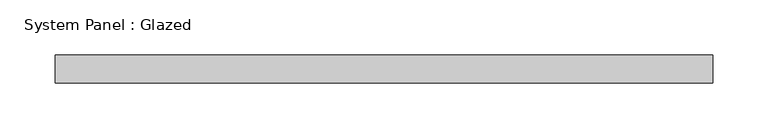
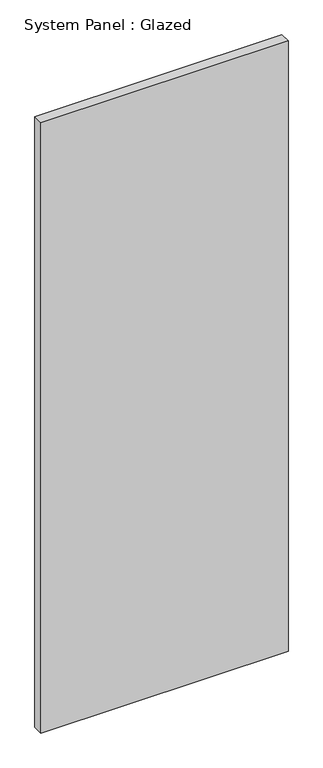
"""IFC4 building model written with IfcOpenShell, lengths in millimetres: plate geometry, System Panel : Glazed."""

from ifc_helpers import new_model, si_unit, origin, origin_with_axes, place, context, project, spatial, polyline, outline, extrude, source, transform, mapped, element, save


def system_panel_glazed_c50c6dba(model_context):
    return source(origin(), model_context, "Body", "SweptSolid", [
        extrude(outline(polyline([(298.45, 19.05), (-298.45, 19.05), (-298.45, 44.45), (298.45, 44.45), (298.45, 19.05)])), origin_with_axes(), (0.0, 0.0, 1.0), 1559.2136257),
    ])


if __name__ == "__main__":
    model = new_model("IFC4")
    model_context = context("Model", 3, world=origin())
    ifc_project = project(units=[si_unit("LENGTHUNIT", "METRE", prefix="MILLI")], contexts=[model_context])
    site = spatial("IfcSite", under=ifc_project)
    building = spatial("IfcBuilding", under=site)
    placement = place(None, origin())
    system_panel_glazed_shape = system_panel_glazed_c50c6dba(model_context)
    element("IfcPlate", 1, ObjectType="System Panel : Glazed", at=placement, inside=building, context=model_context, shape_type="MappedRepresentation", body=[
        mapped(system_panel_glazed_shape, transform((0.0, 0.0, 0.0), x_axis=(1.0, 0.0, 0.0), y_axis=(0.0, 1.0, 0.0), z_axis=(0.0, 0.0, 1.0))),
    ])
    save(model, "model.ifc")

# Revit data of these elements
# Type "System Panel : Glazed"
#   Construction Type Id = "GSP4R"
#   Analytic Construction = "1/8 in Pilkington single glazing"
#   Visual Light Transmittance = 0.9
#   Solar Heat Gain Coefficient = 0.86
#   Heat Transfer Coefficient (U) = 1.18115 BTU/(h·ft²·°F)
#   Define Thermal Properties by = 1
# Element 1 (IfcPlate, "System Panel : Glazed")
#   Materials on its faces: "Glass"
# Materials
#   "Glass": class "Glass", colour RGB 0 128 192, transparency 0.75, Description = "Soda Lime Glass", Cost = 0
